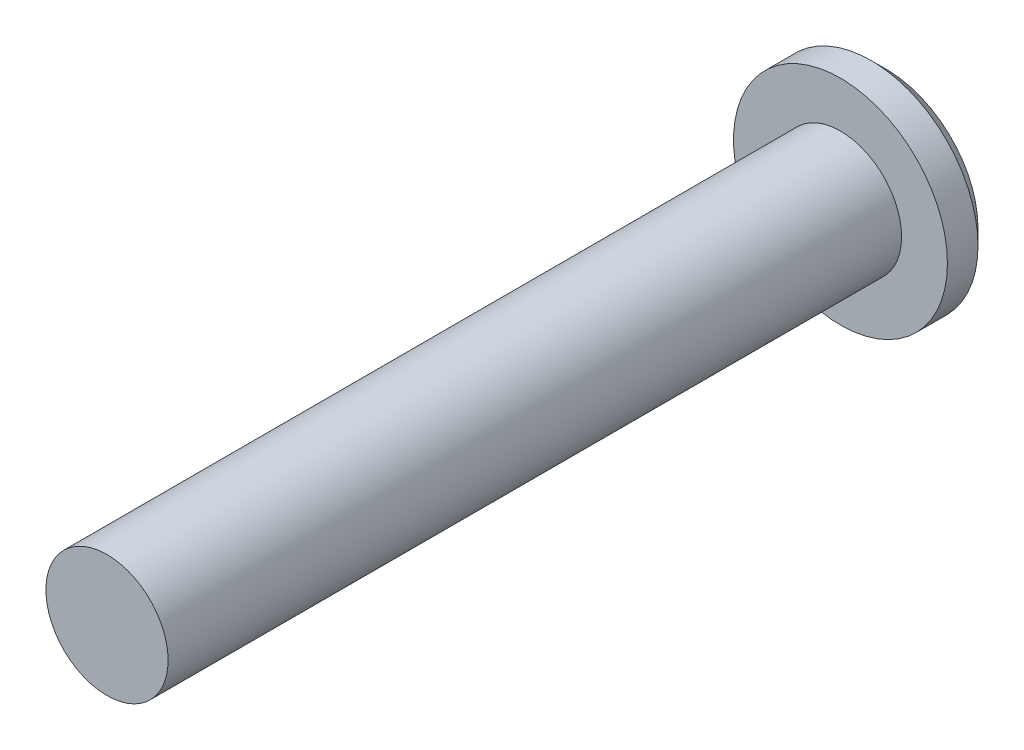
SolidWorks part; units mm, degrees
material "Plain Carbon Steel"
ref_plane "Front Plane" through (0, 0, 0) normal (0, 0, 1) x (1, 0, 0)
ref_plane "Top Plane" through (0, 0, 0) normal (0, 1, 0) x (1, 0, 0)
ref_plane "Right Plane" through (0, 0, 0) normal (1, 0, 0) x (0, 0, -1)
sketch "Head Profile Ø14" plane through (0, 0, 0) normal (0, 0, 1) x (1, 0, 0)
  circle A0 centre (0, 0) radius 7
  dimension "D1" = 14
extrude "Head Ø14x3" add sketch "Head Profile Ø14" along normal blind 3
sketch "Shank Profile Ø8" plane through (0, 0, 3) normal (0, 0, 1) x (1, 0, 0)
  circle A0 centre (0, 0) radius 4
  dimension "D1" = 8
extrude "Shank Ø8x48" add sketch "Shank Profile Ø8" along normal blind 48
cosmetic thread "Cosmetic Thread1" parameters "D1"=3, "D2"=6.561
chamfer "Head Chamfer 1x45°" distance 1 angle 45 1 edges at (7, 0, 0)
